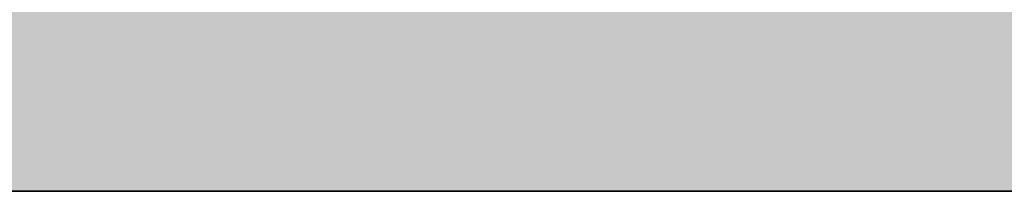
# Model space of a CAD drawing. Units: inches. Extents: x 2083 to 3317, y 1141 to 2115.
# Tile 138 of 256: x 3126.1318 to 3126.6699, y 1263.2614 to 1263.3548. Entities that reach past the tile are written whole.
import ezdxf

# ---------------------------------------------------------------- set-up
doc = ezdxf.new("R2010")
doc.units = ezdxf.units.IN
doc.layers.add('A-ANNO-DIMS', color=2, linetype='Continuous', lineweight=18)
doc.layers.add('A-WALL', color=7, linetype='Continuous', lineweight=35)
doc.layers.add('A-WALL-PATT', color=251, linetype='Continuous', lineweight=13, true_color=0x636466)
doc.styles.get("Standard").update_dxf_attribs({"font": 'arial.ttf'})
doc.dimstyles.new('ISO-25', dxfattribs={"dimtxt": 12, "dimasz": 12, "dimexe": 1.25, "dimexo": 0.625, "dimtad": 1, "dimlunit": 3, "dimtxsty": 'Standard', "dimcen": 2.5, "dimadec": 0, "dimazin": 0, "dimtfac": 1, "dimtmove": 0, "dimatfit": 3, "dimfxl": 1, "dimarcsym": 0})

# ---------------------------------------------------------------- blocks, each defined once
blk = doc.blocks.new('*D10')
at = {"layer": 'A-ANNO-DIMS', "color": 0, "lineweight": -2, "transparency": 16777216}
for p, q in [((2862.95978, 1262.63636), (2862.95978, 1201.38445)), ((3126.95978, 1262.63636), (3126.95978, 1201.38445)), ((2874.95978, 1202.63445), (3114.95978, 1202.63445))]:
    blk.add_line(p, q, dxfattribs=at)
at = {"layer": 'A-ANNO-DIMS', "color": 0, "transparency": 16777216}
for points in [[(2874.95978, 1204.63445), (2874.95978, 1200.63445), (2862.95978, 1202.63445)], [(3114.95978, 1204.63445), (3114.95978, 1200.63445), (3126.95978, 1202.63445)]]:
    blk.add_solid(points, dxfattribs=at)
at = {"layer": 'Defpoints', "color": 0, "transparency": 16777216}
for p in [(2862.95978, 1263.26136), (3126.95978, 1263.26136), (3126.95978, 1202.63445)]:
    blk.add_point(p, dxfattribs=at)
at = {"layer": 'A-ANNO-DIMS', "color": 0, "transparency": 16777216, "insert": (2994.95978, 1209.28401), "char_height": 12, "attachment_point": 5}
blk.add_mtext("22'", dxfattribs=at)
blk = doc.blocks.new('*D26')
at = {"layer": 'A-ANNO-DIMS', "color": 0, "lineweight": -2, "transparency": 16777216}
for p, q in [((3088.98584, 1274.91509), (3088.98584, 1270.95196)), ((3111.24004, 1274.91509), (3111.24004, 1270.95196)), ((3076.98584, 1272.20196), (2840.26245, 1272.20196)), ((3111.24004, 1272.20196), (3088.98584, 1272.20196)), ((3123.24004, 1272.20196), (3135.24004, 1272.20196))]:
    blk.add_line(p, q, dxfattribs=at)
at = {"layer": 'A-ANNO-DIMS', "color": 0, "transparency": 16777216}
for points in [[(3076.98584, 1274.20196), (3076.98584, 1270.20196), (3088.98584, 1272.20196)], [(3123.24004, 1274.20196), (3123.24004, 1270.20196), (3111.24004, 1272.20196)]]:
    blk.add_solid(points, dxfattribs=at)
at = {"layer": 'Defpoints', "color": 0, "transparency": 16777216}
for p in [(3088.98584, 1275.54009), (3111.24004, 1275.54009), (3088.98584, 1272.20196)]:
    blk.add_point(p, dxfattribs=at)
at = {"layer": 'A-ANNO-DIMS', "color": 0, "transparency": 16777216, "insert": (2952.62415, 1279.0316), "char_height": 12, "attachment_point": 5}
blk.add_mtext('NIGHTSTAND 1\'-10 1/2" TYP.', dxfattribs=at)
blk = doc.blocks.new('*D27')
at = {"layer": 'A-ANNO-DIMS', "color": 0, "lineweight": -2, "transparency": 16777216}
for p, q in [((3114.57817, 1309.79428), (3114.57817, 1321.79428)), ((3111.86504, 1297.79428), (3115.82817, 1297.79428)), ((3114.57817, 1297.79428), (3114.57817, 1275.54009)), ((3111.86504, 1275.54009), (3115.82817, 1275.54009)), ((3114.57817, 1263.54009), (3114.57817, 1140.98859))]:
    blk.add_line(p, q, dxfattribs=at)
at = {"layer": 'A-ANNO-DIMS', "color": 0, "transparency": 16777216}
for points in [[(3112.57817, 1309.79428), (3116.57817, 1309.79428), (3114.57817, 1297.79428)], [(3112.57817, 1263.54009), (3116.57817, 1263.54009), (3114.57817, 1275.54009)]]:
    blk.add_solid(points, dxfattribs=at)
at = {"layer": 'Defpoints', "color": 0, "transparency": 16777216}
for p in [(3111.24004, 1297.79428), (3111.24004, 1275.54009), (3114.57817, 1275.54009)]:
    blk.add_point(p, dxfattribs=at)
at = {"layer": 'A-ANNO-DIMS', "color": 0, "transparency": 16777216, "insert": (3107.74853, 1196.26434), "char_height": 12, "attachment_point": 5, "rotation": 90}
blk.add_mtext('1\'-10 1/2" TYP.', dxfattribs=at)

msp = doc.modelspace()

# ---------------------------------------------------------------- hatches: boundary and pattern name
at = {"layer": 'A-WALL-PATT'}
h = msp.add_hatch(color=256, dxfattribs=at)
h.dxf.hatch_style = 1
h.paths.add_polyline_path([(3126.95978, 2020.76136), (2748.95978, 2020.76136), (2604.95978, 2020.76136), (2226.95978, 2020.76136), (2226.95978, 1702.76136), (2466.95978, 1702.76136), (2466.95978, 1582.76136), (2418.95978, 1582.76136), (2418.95978, 1477.76136), (2226.95978, 1477.76136), (2226.95978, 1263.26136), (2544.95978, 1263.26136), (2544.95978, 1411.76136), (2604.95978, 1411.76136), (2685.95978, 1411.76136), (2685.95978, 1420.76136), (2604.95978, 1420.76136), (2604.95978, 1573.76136), (2604.95978, 1702.76136), (2604.95978, 2011.76136), (2748.95978, 2011.76136), (2748.95978, 1702.76136), (2862.95978, 1702.76136), (2862.95978, 1621.76136), (2871.95978, 1621.76136), (2871.95978, 1702.76136), (2883.95978, 1702.76136), (2883.95978, 1706.93946, -0.026459), (2883.95978, 1711.76136), (2757.95978, 1711.76136), (2757.95978, 1807.76136), (2787.95978, 1807.76136), (2787.95978, 1812.26136), (2757.95978, 1812.26136), (2757.95978, 2011.76136), (2877.95978, 2011.76136), (2877.95978, 1812.26136), (2847.95978, 1812.26136), (2847.95978, 1807.76136), (2889.83574, 1807.76136), (2889.83574, 1812.26136), (2882.45978, 1812.26136), (2882.45978, 2011.76136), (3117.95978, 2011.76136), (3117.95978, 1812.26136), (2937.83574, 1812.26136), (2937.83574, 1807.76136), (2995.70978, 1807.76136), (2995.70978, 1796.11767), (3000.20978, 1796.11767), (3000.20978, 1807.76136), (3117.95978, 1807.76136), (3117.95978, 1711.76136), (3000.20978, 1711.76136), (3000.20978, 1760.11767), (2998.5727, 1760.11767, -0.020711), (2995.70978, 1760.11767), (2995.70978, 1711.76136), (2931.95978, 1711.76136), (2931.95978, 1702.76136), (3126.95978, 1702.76136)])
h.paths.add_polyline_path([(2471.45978, 2011.76136), (2471.45978, 1810.01136), (2462.71694, 1810.01136), (2462.71694, 1805.51136), (2505.95978, 1805.51136), (2505.95978, 1810.01136), (2475.95978, 1810.01136), (2475.95978, 2011.76136), (2595.95978, 2011.76136), (2595.95978, 1810.01136), (2565.95978, 1810.01136), (2565.95978, 1805.51136), (2595.95978, 1805.51136), (2595.95978, 1711.76136), (2235.95978, 1711.76136), (2235.95978, 1805.51136), (2353.70978, 1805.51136), (2353.70978, 1796.05416), (2358.20978, 1796.05416), (2358.20978, 1805.51136), (2414.71694, 1805.51136), (2414.71694, 1810.01136), (2235.95978, 1810.01136), (2235.95978, 2011.76136)], flags=16)
h.paths.add_polyline_path([(2270.20473, 1994.61001), (2270.20473, 1970.61001), (2246.20473, 1970.61001), (2246.20473, 1994.61001)], flags=0)
edge = h.paths.add_edge_path(flags=0)
edge.add_ellipse((2332.02739, 1899.79818), major_axis=(-3.04299, 3.04299), ratio=0.1682525, start_angle=-161.33217, end_angle=-156.30711, ccw=False)
edge.add_ellipse((2333.08204, 1898.74353), major_axis=(-1.05465, 1.05465), ratio=0.4535321, start_angle=-123.37102, end_angle=-94.15911)
edge = h.paths.add_edge_path(flags=0)
edge.add_ellipse((2332.02739, 1968.87629), major_axis=(3.04299, 3.04299), ratio=0.1682525, start_angle=18.66783, end_angle=23.69289)
edge.add_spline(control_points=[(2332.9256, 1970.6911), (2332.22677, 1970.3361), (2330.89371, 1969.65891), (2328.41308, 1970.93214), (2327.20393, 1967.74871), (2324.7096, 1969.95559), (2322.53282, 1967.01235), (2320.01285, 1971.29581), (2317.68031, 1968.15784), (2316.04053, 1967.10205), (2315.4269, 1966.8096)], knot_values=[0, 0, 0, 0, 2.267059, 4.324559, 6.685584, 8.878641, 11.121502, 14.300359, 17.755284, 19.732645, 19.732645, 19.732645, 19.732645], degree=3, periodic=0)
edge.add_ellipse((2332.02739, 1968.87629), major_axis=(3.04299, 3.04299), ratio=0.1682525, start_angle=18.66783, end_angle=23.69289, ccw=False)
edge.add_ellipse((2333.08204, 1969.93094), major_axis=(1.05465, 1.05465), ratio=0.4535321, start_angle=56.62898, end_angle=85.84089, ccw=False)
edge = h.paths.add_edge_path(flags=0)
edge.add_spline(control_points=[(2296.42829, 1967.98791), (2293.6278, 1965.33631), (2287.70362, 1959.72709), (2299.74386, 1949.9957), (2294.53259, 1935.66853), (2290.57323, 1920.60351), (2293.39412, 1909.97369), (2296.18541, 1904.96654)], knot_values=[0.099185, 0.099185, 0.099185, 0.099185, 0.345301, 0.619822, 0.982653, 1.386093, 1.810555, 1.810555, 1.810555, 1.810555], degree=3, periodic=0)
edge.add_spline(control_points=[(2296.18541, 1904.96654), (2297.38358, 1902.6193), (2298.00097, 1901.94931), (2298.55297, 1901.46815)], knot_values=[0.006246, 0.006246, 0.006246, 0.006246, 0.055476, 0.055476, 0.055476, 0.055476], degree=3, periodic=0)
edge.add_spline(control_points=[(2298.55297, 1901.46815), (2297.25861, 1900.92322), (2295.22529, 1900.23213), (2293.06023, 1900.61421), (2292.10142, 1900.78841), (2292.08958, 1900.79057)], knot_values=[0.312835, 0.312835, 0.312835, 0.312835, 0.40178, 0.474987, 0.475903, 0.475903, 0.475903, 0.475903], degree=3, periodic=0)
edge.add_arc((2292.79365, 1904.66411), 3.93701, 215.4209, 259.69818, ccw=False)
edge.add_spline(control_points=[(2289.58531, 1902.3823), (2289.47665, 1902.53509), (2289.36848, 1902.68804), (2289.26086, 1902.84117)], knot_values=[0.102872, 0.102872, 0.102872, 0.102872, 0.116896, 0.116896, 0.116896, 0.116896], degree=3, periodic=0)
edge.add_spline(control_points=[(2289.26086, 1902.84117), (2288.6866, 1902.55019), (2287.64005, 1902.0199), (2285.88134, 1901.87395), (2283.85297, 1901.50435), (2281.71999, 1899.71054), (2278.46699, 1899.49294), (2276.15714, 1901.8832), (2272.25895, 1899.80407), (2267.77761, 1901.84318), (2262.24388, 1900.18403), (2257.41493, 1901.78206), (2254.31837, 1900.72612), (2253.17828, 1900.33734)], knot_values=[0, 0, 0, 0, 1.907977, 3.477176, 5.261074, 7.972851, 11.680248, 13.717921, 16.939592, 22.789562, 27.502503, 33.595215, 37.145618, 37.145618, 37.145618, 37.145618], degree=3, periodic=0)
edge.add_line((2253.17828, 1900.33734), (2250.24424, 1902.84117))
edge.add_line((2250.24424, 1902.84117), (2250.24424, 1965.8333))
edge.add_line((2250.24424, 1965.8333), (2253.17828, 1968.33712))
edge.add_spline(control_points=[(2253.17828, 1968.33712), (2254.31837, 1967.94835), (2257.41493, 1966.89241), (2262.24388, 1968.49043), (2267.77761, 1966.83128), (2271.52673, 1968.53722), (2273.87591, 1967.82829), (2274.2067, 1967.72764)], knot_values=[0, 0, 0, 0, 0.09018, 0.244935, 0.364644, 0.513233, 0.537855, 0.537855, 0.537855, 0.537855], degree=3, periodic=0)
edge.add_arc((2274.35289, 1963.79335), 3.93701, 72.05113, 92.12795, ccw=False)
edge.add_arc((2281.29693, 1985.23), 18.5963, 252.051134, 288.565722)
edge.add_arc((2292.31672, 1956.02888), 12.64608, 71.026788, 113.778218, ccw=False)
edge = h.paths.add_edge_path(flags=0)
edge.add_spline(control_points=[(2274.89941, 1951.85619), (2275.06616, 1951.61659), (2275.23269, 1951.37659), (2275.39799, 1951.13585)], knot_values=[1.409916, 1.409916, 1.409916, 1.409916, 1.43159, 1.43159, 1.43159, 1.43159], degree=3, periodic=0)
edge.add_spline(control_points=[(2275.39799, 1951.13585), (2275.79211, 1950.56189), (2276.17923, 1949.98377), (2276.54555, 1949.3971)], knot_values=[1.358238, 1.358238, 1.358238, 1.358238, 1.409916, 1.409916, 1.409916, 1.409916], degree=3, periodic=0)
edge.add_line((2276.54555, 1949.3971), (2277.43729, 1947.86218))
edge.add_spline(control_points=[(2277.43729, 1947.86218), (2276.30383, 1945.67311), (2274.6397, 1942.42688), (2274.63161, 1938.0939), (2272.79912, 1930.85155), (2274.35643, 1943.89705), (2275.94768, 1947.92336), (2276.54555, 1949.3971)], knot_values=[0.005632, 0.005632, 0.005632, 0.005632, 0.186014, 0.266002, 0.357087, 0.59639, 0.739732, 0.739732, 0.739732, 0.739732], degree=3, periodic=0)
edge.add_spline(control_points=[(2276.54555, 1949.3971), (2276.17923, 1949.98377), (2275.79211, 1950.56189), (2275.39799, 1951.13585)], knot_values=[1.358238, 1.358238, 1.358238, 1.358238, 1.409916, 1.409916, 1.409916, 1.409916], degree=3, periodic=0)
edge.add_spline(control_points=[(2275.39799, 1951.13585), (2274.9425, 1950.08045), (2274.20776, 1948.02527), (2273.9346, 1944.85148), (2272.46853, 1937.62749), (2273.46622, 1945.69647), (2274.70062, 1951.05947), (2274.89941, 1951.85619)], knot_values=[0.104364, 0.104364, 0.104364, 0.104364, 0.189636, 0.269624, 0.36071, 0.600013, 0.644622, 0.644622, 0.644622, 0.644622], degree=3, periodic=0)
h.paths.add_polyline_path([(2269.16751, 1963.12757, -0.357527), (2268.17063, 1960.97637, -0.092561), (2268.17063, 1939.43632, -0.357527), (2269.16751, 1937.28512, -0.357527), (2267.01631, 1938.282, -0.164785), (2254.68558, 1938.282, -0.357527), (2252.53438, 1937.28512, -0.357527), (2253.53126, 1939.43632, -0.092561), (2253.53126, 1960.97637, -0.357527), (2252.53438, 1963.12757, -0.357527), (2254.68558, 1962.13069, -0.164785), (2267.01631, 1962.13069, -0.357527)], flags=0)
h.paths.add_polyline_path([(2248.87407, 1967.8018), (2248.87407, 1957.02771), (2249.45778, 1957.02771), (2249.45778, 1911.64676), (2248.87407, 1911.64676), (2248.87407, 1900.87267), (2246.51186, 1900.87267, 0.197327), (2244.14966, 1902.45687), (2244.14966, 1966.21759, 0.197327), (2246.51186, 1967.8018)], flags=0)
h.paths.add_polyline_path([(2269.16751, 1931.38934, -0.357527), (2268.17063, 1929.23814, -0.092561), (2268.17063, 1907.6981, -0.357527), (2269.16751, 1905.54689, -0.357527), (2267.01631, 1906.54377, -0.164785), (2254.68558, 1906.54377, -0.357527), (2252.53438, 1905.54689, -0.357527), (2253.53126, 1907.6981, -0.092561), (2253.53126, 1929.23814, -0.357527), (2252.53438, 1931.38934, -0.357527), (2254.68558, 1930.39246, -0.164785), (2267.01631, 1930.39246, -0.357527)], flags=0)
edge = h.paths.add_edge_path(flags=0)
edge.add_spline(control_points=[(2276.19686, 1906.7237), (2276.16814, 1909.02893), (2276.11405, 1913.37185), (2270.59842, 1924.92498), (2273.90517, 1919.01278), (2275.92171, 1916.26206), (2275.47457, 1912.40215), (2277.25787, 1910.38062), (2276.69604, 1908.22504), (2276.64622, 1906.81302), (2276.61782, 1906.00841)], knot_values=[0, 0, 0, 0, 8.61026, 16.221274, 18.843057, 23.804898, 27.440828, 29.356102, 31.203478, 33.650687, 33.650687, 33.650687, 33.650687], degree=3, periodic=0)
edge.add_spline(control_points=[(2276.61782, 1906.00841), (2276.62331, 1905.62414), (2276.49774, 1904.62866), (2275.44178, 1903.85473), (2274.93731, 1903.08045), (2274.85908, 1902.84117)], knot_values=[0.156488, 0.156488, 0.156488, 0.156488, 0.184398, 0.231376, 0.250598, 0.250598, 0.250598, 0.250598], degree=3, periodic=0)
edge.add_line((2274.85908, 1902.84117), (2276.50598, 1902.84117))
edge.add_spline(control_points=[(2276.50598, 1902.84117), (2276.78831, 1903.08494), (2277.66507, 1904.1252), (2278.24954, 1904.34074), (2277.65387, 1908.52739), (2278.15567, 1906.22781), (2278.10046, 1905.28595), (2278.84667, 1904.06901), (2277.85679, 1903.41495), (2277.87419, 1902.99105), (2277.90356, 1902.84117)], knot_values=[0.059574, 0.059574, 0.059574, 0.059574, 0.080753, 0.103741, 0.16972, 0.176036, 0.207137, 0.240474, 0.262341, 0.27366, 0.27366, 0.27366, 0.27366], degree=3, periodic=0)
edge.add_line((2277.90356, 1902.84117), (2280.02983, 1902.84117))
edge.add_spline(control_points=[(2280.02983, 1902.84117), (2279.88822, 1903.0884), (2279.49926, 1903.98155), (2280.15228, 1905.93935), (2278.10362, 1909.65776), (2279.76239, 1907.18529), (2280.3279, 1904.87486), (2280.48511, 1903.48959), (2281.46327, 1903.24943), (2281.75834, 1902.9365), (2281.83404, 1902.84117)], knot_values=[0.013856, 0.013856, 0.013856, 0.013856, 0.034874, 0.088867, 0.107879, 0.126738, 0.158714, 0.193757, 0.217487, 0.226722, 0.226722, 0.226722, 0.226722], degree=3, periodic=0)
edge.add_spline(control_points=[(2281.83404, 1902.84117), (2281.78753, 1902.8267), (2281.64702, 1902.78299), (2281.39553, 1902.85949), (2281.08808, 1902.98524), (2280.72068, 1903.0609), (2280.33345, 1903.02573), (2280.12477, 1902.89888), (2280.02983, 1902.84117)], knot_values=[0, 0, 0, 0, 0.14413, 0.435517, 0.749276, 1.153046, 1.548371, 1.878348, 1.878348, 1.878348, 1.878348], degree=3, periodic=0)
edge.add_line((2280.02983, 1902.84117), (2277.90356, 1902.84117))
edge.add_spline(control_points=[(2277.90356, 1902.84117), (2277.89286, 1902.79586), (2277.8654, 1902.67964), (2277.60748, 1902.68748), (2277.27405, 1902.8007), (2276.83792, 1902.61977), (2276.58381, 1902.78926), (2276.50598, 1902.84117)], knot_values=[0, 0, 0, 0, 0.127189, 0.326199, 0.628009, 1.24357, 1.515331, 1.515331, 1.515331, 1.515331], degree=3, periodic=0)
edge.add_line((2276.50598, 1902.84117), (2274.85908, 1902.84117))
edge.add_spline(control_points=[(2274.85908, 1902.84117), (2274.81444, 1902.89859), (2274.72513, 1903.01345), (2274.49348, 1903.11897), (2274.24429, 1902.96054), (2273.93712, 1903.18494), (2273.61404, 1902.98314), (2273.40832, 1902.88304), (2273.32225, 1902.84117)], knot_values=[0, 0, 0, 0, 0.21843, 0.436957, 0.687977, 0.990379, 1.398396, 1.69185, 1.69185, 1.69185, 1.69185], degree=3, periodic=0)
edge.add_spline(control_points=[(2273.32225, 1902.84117), (2273.61674, 1903.44569), (2274.274, 1904.53825), (2276.02724, 1904.5737), (2276.20696, 1906.58364), (2276.19686, 1906.7237)], knot_values=[0.012227, 0.012227, 0.012227, 0.012227, 0.059472, 0.106218, 0.134458, 0.134458, 0.134458, 0.134458], degree=3, periodic=0)
h.paths.add_polyline_path([(2270.77605, 1897.78983), (2270.77605, 1873.78983), (2246.77605, 1873.78983), (2246.77605, 1897.78983)], flags=0)
h.paths.add_polyline_path([(2353.70978, 1760.00506), (2353.70978, 1760.05416), (2358.20978, 1760.05416, -0.033729)], flags=0)
h.paths.add_polyline_path([(2321.81912, 1737.52919), (2341.99533, 1737.52919, -0.414214), (2343.20327, 1736.32124), (2343.20327, 1721.0206, -0.414214), (2341.99533, 1719.81265), (2321.81912, 1719.81265, -0.414214), (2320.61117, 1721.0206), (2320.61117, 1736.32124, -0.414214)], flags=0)
h.paths.add_polyline_path([(2324.23501, 1736.32124), (2339.57944, 1736.32124, -0.414214), (2341.99533, 1733.90535), (2341.99533, 1725.44973, -0.414214), (2339.57944, 1723.03384), (2333.68059, 1723.03384), (2333.84532, 1722.04547, -0.870646), (2335.4254, 1721.82589, -0.767327), (2333.92269, 1721.42324), (2331.29102, 1721.42324, -0.767327), (2329.78832, 1721.82589, -0.870646), (2331.3684, 1722.04547), (2331.53313, 1723.03384), (2324.23501, 1723.03384, -0.414214), (2321.81912, 1725.44973), (2321.81912, 1733.90535, -0.414214)], flags=0)
h.paths.add_polyline_path([(2570.48379, 1928.61544), (2589.68379, 1928.61544), (2590.16883, 1928.61544), (2590.16883, 1904.9934), (2570.48379, 1904.9934)], flags=0)
h.paths.add_polyline_path([(2574.44732, 1927.26382, -1), (2572.82884, 1927.26382, -1)], flags=0)
h.paths.add_polyline_path([(2573.08987, 1926.94088), (2573.92503, 1927.77604), (2574.14774, 1927.55333), (2573.31258, 1926.71817)], flags=0)
h.paths.add_polyline_path([(2578.77906, 1919.72962, -1), (2571.59166, 1919.72962, -1)], flags=0)
h.paths.add_polyline_path([(2578.38536, 1919.72962, -1), (2571.98536, 1919.72962, -1)], flags=0)
h.paths.add_polyline_path([(2331.59576, 1729.47622, -1), (2333.61795, 1729.47622, -1)], flags=0)
h.paths.add_polyline_path([(2578.03423, 1927.26382, -1), (2576.41574, 1927.26382, -1)], flags=0)
h.paths.add_polyline_path([(2576.68885, 1927.53109), (2576.91156, 1927.7538), (2577.74673, 1926.91863), (2577.52402, 1926.69592)], flags=0)
h.paths.add_polyline_path([(2578.13906, 1909.85954, -1), (2572.23166, 1909.85954, -1)], flags=0)
h.paths.add_polyline_path([(2577.74536, 1909.85954, -1), (2572.62536, 1909.85954, -1)], flags=0)
h.paths.add_polyline_path([(2583.79772, 1927.26382, -1), (2582.17923, 1927.26382, -1)], flags=0)
h.paths.add_polyline_path([(2582.71865, 1927.7538), (2583.55381, 1926.91863), (2583.3311, 1926.69592), (2582.49594, 1927.53109)], flags=0)
h.paths.add_polyline_path([(2582.49594, 1927.53109), (2582.71865, 1927.7538), (2583.55381, 1926.91863), (2583.3311, 1926.69592)], flags=0)
h.paths.add_polyline_path([(2587.73906, 1920.52962, -1), (2581.83166, 1920.52962, -1)], flags=0)
h.paths.add_polyline_path([(2587.34536, 1920.52962, -1), (2582.22536, 1920.52962, -1)], flags=0)
h.paths.add_polyline_path([(2587.38462, 1927.26382, -1), (2585.76613, 1927.26382, -1)], flags=0)
h.paths.add_polyline_path([(2586.08199, 1926.98025), (2586.91716, 1927.81541), (2587.13987, 1927.5927), (2586.3047, 1926.75754)], flags=0)
h.paths.add_polyline_path([(2588.37906, 1910.65954, -1), (2581.19166, 1910.65954, -1)], flags=0)
h.paths.add_polyline_path([(2587.98536, 1910.65954, -1), (2581.58536, 1910.65954, -1)], flags=0)
h.paths.add_polyline_path([(2417.16773, 1729.4779), (2437.34394, 1729.4779, -0.414214), (2438.55188, 1728.26995), (2438.55188, 1712.96931, -0.414214), (2437.34394, 1711.76136), (2417.16773, 1711.76136, -0.414214), (2415.95978, 1712.96931), (2415.95978, 1728.26995, -0.414214)], flags=0)
h.paths.add_polyline_path([(2419.58362, 1728.26995), (2434.92805, 1728.26995, -0.414214), (2437.34394, 1725.85406), (2437.34394, 1717.39844, -0.414214), (2434.92805, 1714.98255), (2429.0292, 1714.98255), (2429.19393, 1713.99418, -0.870646), (2430.77401, 1713.7746, -0.767327), (2429.2713, 1713.37195), (2426.63963, 1713.37195, -0.767327), (2425.13693, 1713.7746, -0.870646), (2426.71701, 1713.99418), (2426.88174, 1714.98255), (2419.58362, 1714.98255, -0.414214), (2417.16773, 1717.39844), (2417.16773, 1725.85406, -0.414214)], flags=0)
h.paths.add_polyline_path([(2419.58362, 1728.26995), (2434.92805, 1728.26995, -0.414214), (2437.34394, 1725.85406), (2437.34394, 1717.39844, -0.414214), (2434.92805, 1714.98255), (2429.0292, 1714.98255), (2428.35812, 1719.00903), (2427.55282, 1719.00903), (2426.88174, 1714.98255), (2419.58362, 1714.98255, -0.414214), (2417.16773, 1717.39844), (2417.16773, 1725.85406, -0.414214)], flags=0)
h.paths.add_polyline_path([(2426.94437, 1721.42492, -1), (2428.96656, 1721.42492, -1)], flags=0)
h.paths.add_polyline_path([(2475.95978, 1702.76136), (2595.95978, 1702.76136), (2595.95978, 1582.76136), (2475.95978, 1582.76136)], flags=16)
h.paths.add_polyline_path([(2427.95978, 1573.76136), (2595.95978, 1573.76136), (2595.95978, 1468.76136), (2595.95978, 1420.76136), (2384.45978, 1420.76136), (2384.45978, 1468.76136), (2427.95978, 1468.76136)], flags=16)
h.paths.add_polyline_path([(2379.95978, 1468.76136), (2379.95978, 1420.76136), (2235.95978, 1420.76136), (2235.95978, 1468.76136)], flags=16)
h.paths.add_polyline_path([(2317.816, 1466.69577), (2337.9922, 1466.69577, -0.414214), (2339.20015, 1465.48782), (2339.20015, 1450.18718, -0.414214), (2337.9922, 1448.97923), (2317.816, 1448.97923, -0.414214), (2316.60805, 1450.18718), (2316.60805, 1465.48782, -0.414214)], flags=0)
h.paths.add_polyline_path([(2320.23189, 1465.48782), (2335.57631, 1465.48782, -0.414214), (2337.9922, 1463.07193), (2337.9922, 1454.61631, -0.414214), (2335.57631, 1452.20042), (2329.67747, 1452.20042), (2329.84219, 1451.21205, -0.870646), (2331.42228, 1450.99247, -0.767327), (2329.91957, 1450.58983), (2327.2879, 1450.58983, -0.767327), (2325.7852, 1450.99247, -0.870646), (2327.36528, 1451.21205), (2327.53001, 1452.20042), (2320.23189, 1452.20042, -0.414214), (2317.816, 1454.61631), (2317.816, 1463.07193, -0.414214)], flags=0)
h.paths.add_polyline_path([(2320.23189, 1465.48782), (2335.57631, 1465.48782, -0.414214), (2337.9922, 1463.07193), (2337.9922, 1454.61631, -0.414214), (2335.57631, 1452.20042), (2329.67747, 1452.20042), (2329.00638, 1456.22691), (2328.20109, 1456.22691), (2327.53001, 1452.20042), (2320.23189, 1452.20042, -0.414214), (2317.816, 1454.61631), (2317.816, 1463.07193, -0.414214)], flags=0)
h.paths.add_polyline_path([(2327.59264, 1458.6428, -1), (2329.61483, 1458.6428, -1)], flags=0)
h.paths.add_polyline_path([(2244.41174, 1433.34045), (2241.92094, 1433.34045, -0.414214), (2240.01786, 1435.24354), (2240.01786, 1440.95281, -0.414211), (2241.92093, 1442.8559), (2244.41174, 1442.8559, -1.976472)], flags=0)
h.paths.add_polyline_path([(2245.35689, 1434.39754, -0.414214), (2245.35689, 1441.79881, -2.144098)], flags=0)
h.paths.add_polyline_path([(2535.95978, 1416.26136), (2535.95978, 1272.26136), (2235.95978, 1272.26136), (2235.95978, 1416.26136)], flags=16)
h.paths.add_polyline_path([(2260.11956, 1384.29284), (2260.11956, 1362.03865), (2237.86537, 1362.03865), (2237.86537, 1384.29284)], flags=0)
edge = h.paths.add_edge_path(flags=0)
edge.add_line((2318.25185, 1362.0933), (2318.1458, 1362.00097))
edge.add_ellipse((2317.44512, 1360.43104), major_axis=(2.82164, 2.82164), ratio=0.1682525, start_angle=18.66783, end_angle=20.94813, ccw=False)
edge.add_ellipse((2318.42305, 1361.40897), major_axis=(0.97793, 0.97793), ratio=0.4535321, start_angle=56.62898, end_angle=70.2262, ccw=False)
edge = h.paths.add_edge_path(flags=0)
edge.add_line((2319.10737, 1295.57108), (2319.01504, 1295.67713))
edge.add_ellipse((2317.44512, 1296.37781), major_axis=(-2.82164, 2.82164), ratio=0.1682525, start_angle=-161.33217, end_angle=-159.05187, ccw=False)
edge.add_ellipse((2318.42305, 1295.39988), major_axis=(-0.97793, 0.97793), ratio=0.4535321, start_angle=-123.37102, end_angle=-109.7738)
edge = h.paths.add_edge_path(flags=0)
edge.add_spline(control_points=[(2284.21035, 1301.17022), (2284.58069, 1300.44472), (2284.89119, 1299.89202), (2285.15955, 1299.46102)], knot_values=[0.039066, 0.039066, 0.039066, 0.039066, 0.055476, 0.055476, 0.055476, 0.055476], degree=3, periodic=0)
edge.add_line((2285.15955, 1299.46102), (2284.21035, 1301.17022))
edge = h.paths.add_edge_path(flags=0)
edge.add_line((2280.41246, 1297.29801), (2283.36999, 1297.03612))
edge.add_line((2283.36999, 1297.03612), (2286.40569, 1297.92631))
edge.add_spline(control_points=[(2286.40569, 1297.92631), (2285.30549, 1297.46312), (2284.34478, 1297.12915), (2283.36999, 1297.03612)], knot_values=[0.394369, 0.394369, 0.394369, 0.394369, 0.475903, 0.475903, 0.475903, 0.475903], degree=3, periodic=0)
edge.add_spline(control_points=[(2283.36999, 1297.03612), (2283.28139, 1297.02767), (2282.31629, 1296.95734), (2281.3125, 1297.13448), (2280.42344, 1297.29602), (2280.41246, 1297.29801)], knot_values=[0.312835, 0.312835, 0.312835, 0.312835, 0.320246, 0.393453, 0.394369, 0.394369, 0.394369, 0.394369], degree=3, periodic=0)
edge = h.paths.add_edge_path(flags=0)
edge.add_line((2284.43556, 1359.60729), (2280.44629, 1355.32805))
edge.add_line((2280.44629, 1355.32805), (2279.57999, 1351.01775))
edge.add_line((2279.57999, 1351.01775), (2282.41297, 1346.58043))
edge.add_spline(control_points=[(2282.41297, 1346.58043), (2283.15333, 1345.58924), (2284.2529, 1344.0289), (2284.80104, 1342.38717), (2284.93516, 1341.80554)], knot_values=[1.240098, 1.240098, 1.240098, 1.240098, 1.332892, 1.382712, 1.382712, 1.382712, 1.382712], degree=3, periodic=0)
edge.add_spline(control_points=[(2284.93516, 1341.80554), (2285.31911, 1340.1406), (2285.23303, 1338.4092), (2284.90994, 1336.65412)], knot_values=[1.097484, 1.097484, 1.097484, 1.097484, 1.240098, 1.240098, 1.240098, 1.240098], degree=3, periodic=0)
edge.add_spline(control_points=[(2284.90994, 1336.65412), (2284.58685, 1334.89904), (2284.02675, 1333.12027), (2283.46264, 1331.36058)], knot_values=[0.95487, 0.95487, 0.95487, 0.95487, 1.097484, 1.097484, 1.097484, 1.097484], degree=3, periodic=0)
edge.add_line((2283.46264, 1331.36058), (2281.89038, 1326.15336))
edge.add_line((2281.89038, 1326.15336), (2280.75626, 1321.05609))
edge.add_line((2280.75626, 1321.05609), (2280.2992, 1316.00198))
edge.add_line((2280.2992, 1316.00198), (2280.71593, 1310.95007))
edge.add_line((2280.71593, 1310.95007), (2282.02809, 1305.97214))
edge.add_line((2282.02809, 1305.97214), (2284.21035, 1301.17022))
edge.add_spline(control_points=[(2284.21035, 1301.17022), (2283.34073, 1302.73019), (2282.6119, 1304.33649), (2282.02809, 1305.97214)], knot_values=[0.099185, 0.099185, 0.099185, 0.099185, 0.241799, 0.241799, 0.241799, 0.241799], degree=3, periodic=0)
edge.add_spline(control_points=[(2282.02809, 1305.97214), (2281.44428, 1307.60778), (2281.00549, 1309.27276), (2280.71593, 1310.95007)], knot_values=[0.241799, 0.241799, 0.241799, 0.241799, 0.384413, 0.384413, 0.384413, 0.384413], degree=3, periodic=0)
edge.add_spline(control_points=[(2280.71593, 1310.95007), (2280.43324, 1312.58761), (2280.28939, 1314.27696), (2280.29889, 1315.96203), (2280.2992, 1316.00198)], knot_values=[0.384413, 0.384413, 0.384413, 0.384413, 0.523647, 0.527028, 0.527028, 0.527028, 0.527028], degree=3, periodic=0)
edge.add_spline(control_points=[(2280.2992, 1316.00198), (2280.31233, 1317.68696), (2280.47787, 1319.36793), (2280.75626, 1321.05609)], knot_values=[0.527028, 0.527028, 0.527028, 0.527028, 0.669642, 0.669642, 0.669642, 0.669642], degree=3, periodic=0)
edge.add_spline(control_points=[(2280.75626, 1321.05609), (2281.03465, 1322.74425), (2281.42588, 1324.43961), (2281.89038, 1326.15336)], knot_values=[0.669642, 0.669642, 0.669642, 0.669642, 0.812256, 0.812256, 0.812256, 0.812256], degree=3, periodic=0)
edge.add_spline(control_points=[(2281.89038, 1326.15336), (2282.26438, 1327.53325), (2282.78787, 1329.26181), (2283.35275, 1331.01778), (2283.46264, 1331.36058)], knot_values=[0.812256, 0.812256, 0.812256, 0.812256, 0.927087, 0.95487, 0.95487, 0.95487, 0.95487], degree=3, periodic=0)
edge.add_line((2283.46264, 1331.36058), (2284.90994, 1336.65412))
edge.add_line((2284.90994, 1336.65412), (2284.93516, 1341.80554))
edge.add_line((2284.93516, 1341.80554), (2282.41297, 1346.58043))
edge.add_spline(control_points=[(2282.41297, 1346.58043), (2281.27513, 1348.10379), (2280.07845, 1349.57032), (2279.57999, 1351.01775)], knot_values=[1.382712, 1.382712, 1.382712, 1.382712, 1.525326, 1.525326, 1.525326, 1.525326], degree=3, periodic=0)
edge.add_spline(control_points=[(2279.57999, 1351.01775), (2279.44328, 1351.41472), (2279.13631, 1352.85692), (2279.73519, 1354.29039), (2280.44629, 1355.32805)], knot_values=[1.525326, 1.525326, 1.525326, 1.525326, 1.564439, 1.667941, 1.667941, 1.667941, 1.667941], degree=3, periodic=0)
edge.add_spline(control_points=[(2280.44629, 1355.32805), (2281.42611, 1356.75784), (2282.93084, 1358.18256), (2284.43556, 1359.60729)], knot_values=[1.667941, 1.667941, 1.667941, 1.667941, 1.810555, 1.810555, 1.810555, 1.810555], degree=3, periodic=0)
edge.add_arc((2280.62307, 1348.51818), 11.72618, 71.026788, 113.778218)
edge.add_arc((2270.40489, 1375.59516), 17.24357, 252.051134, 288.565722, ccw=False)
edge.add_arc((2263.96597, 1355.71785), 3.65062, 72.05113, 92.12795)
edge.add_arc((2263.96597, 1355.71785), 3.65062, 92.12795, 177.98513)
edge.add_spline(control_points=[(2260.3176, 1355.8462), (2260.26042, 1354.22067), (2260.55128, 1350.18655), (2262.99934, 1346.76625), (2264.47274, 1344.64902)], knot_values=[1.43159, 1.43159, 1.43159, 1.43159, 1.564144, 1.770695, 1.770695, 1.770695, 1.770695], degree=3, periodic=0)
edge.add_line((2264.47274, 1344.64902), (2264.93559, 1343.98253))
edge.add_spline(control_points=[(2263.80104, 1340.24811), (2263.84324, 1340.51409), (2264.06724, 1341.75647), (2264.51269, 1343.00245), (2264.93505, 1343.98108)], knot_values=[0.53657, 0.53657, 0.53657, 0.53657, 0.559349, 0.644622, 0.644622, 0.644622, 0.644622], degree=3, periodic=0)
edge.add_spline(control_points=[(2264.93505, 1343.98108), (2265.11777, 1343.71497), (2265.29888, 1343.44791), (2265.47676, 1343.17936)], knot_values=[1.384077, 1.384077, 1.384077, 1.384077, 1.409916, 1.409916, 1.409916, 1.409916], degree=3, periodic=0)
edge.add_spline(control_points=[(2265.47676, 1343.17936), (2265.65464, 1342.91082), (2265.8293, 1342.64081), (2265.99913, 1342.36881)], knot_values=[1.358238, 1.358238, 1.358238, 1.358238, 1.384077, 1.384077, 1.384077, 1.384077], degree=3, periodic=0)
edge.add_line((2265.99913, 1342.36881), (2266.82601, 1340.94555))
edge.add_spline(control_points=[(2266.82601, 1340.94555), (2268.8944, 1337.08969), (2271.39817, 1325.843), (2270.51616, 1310.56856), (2275.91938, 1301.86061), (2277.78951, 1299.19945)], knot_values=[0.116896, 0.116896, 0.116896, 0.116896, 0.472987, 1.050969, 1.313793, 1.313793, 1.313793, 1.313793], degree=3, periodic=0)
edge.add_spline(control_points=[(2277.78951, 1299.19945), (2277.83941, 1299.12845), (2277.88943, 1299.0575), (2277.93957, 1298.98658)], knot_values=[0.109884, 0.109884, 0.109884, 0.109884, 0.116896, 0.116896, 0.116896, 0.116896], degree=3, periodic=0)
edge.add_line((2277.93957, 1298.98658), (2277.78885, 1299.19911))
edge.add_spline(control_points=[(2277.78885, 1299.19911), (2277.25658, 1298.92941), (2276.28635, 1298.4379), (2275.03935, 1298.33442), (2274.38333, 1298.2389), (2274.21525, 1298.20934)], knot_values=[33.12187, 33.12187, 33.12187, 33.12187, 35.029056, 36.598255, 37.144827, 37.144827, 37.144827, 37.144827], degree=3, periodic=0)
edge.add_line((2274.21525, 1298.20934), (2273.07315, 1297.89296))
edge.add_spline(control_points=[(2273.07315, 1297.89296), (2272.32294, 1297.57978), (2271.03915, 1296.51051), (2269.24839, 1296.22606), (2268.4231, 1296.37465)], knot_values=[26.532584, 26.532584, 26.532584, 26.532584, 29.198919, 31.839101, 31.839101, 31.839101, 31.839101], degree=3, periodic=0)
edge.add_line((2268.4231, 1296.37465), (2263.8785, 1297.45753))
edge.add_spline(control_points=[(2263.8785, 1297.45753), (2263.55608, 1297.35943), (2261.86031, 1296.83869), (2260.23878, 1297.28241), (2258.93345, 1297.51646)], knot_values=[15.919551, 15.919551, 15.919551, 15.919551, 16.939592, 21.226067, 21.226067, 21.226067, 21.226067], degree=3, periodic=0)
edge.add_line((2258.93345, 1297.51646), (2254.05523, 1297.32901))
edge.add_spline(control_points=[(2254.05523, 1297.32901), (2253.75553, 1297.29582), (2252.11368, 1297.16517), (2250.46187, 1297.54422), (2249.12969, 1297.66788)], knot_values=[5.306517, 5.306517, 5.306517, 5.306517, 6.276435, 10.613034, 10.613034, 10.613034, 10.613034], degree=3, periodic=0)
edge.add_line((2249.12969, 1297.66788), (2244.33165, 1296.87776))
edge.add_line((2244.33165, 1296.87776), (2241.61103, 1299.19945))
edge.add_line((2241.61103, 1299.19945), (2241.61103, 1357.6094))
edge.add_line((2241.61103, 1357.6094), (2244.33165, 1359.9311))
edge.add_line((2244.33165, 1359.9311), (2252.72882, 1359.54269))
edge.add_spline(control_points=[(2252.72882, 1359.54269), (2252.87094, 1359.54644), (2253.30574, 1359.54817), (2253.73984, 1359.51427), (2254.03174, 1359.48243)], knot_values=[0.233291, 0.233291, 0.233291, 0.233291, 0.244935, 0.268927, 0.268927, 0.268927, 0.268927], degree=3, periodic=0)
edge.add_line((2254.03174, 1359.48243), (2259.58719, 1359.41639))
edge.add_spline(control_points=[(2259.58719, 1359.41639), (2260.67707, 1359.6285), (2262.0732, 1359.897), (2263.52369, 1359.45928), (2263.83042, 1359.36595)], knot_values=[0.422516, 0.422516, 0.422516, 0.422516, 0.513233, 0.537855, 0.537855, 0.537855, 0.537855], degree=3, periodic=0)
edge.add_arc((2263.96597, 1355.71785), 3.65062, 72.05113, 92.12795, ccw=False)
edge.add_arc((2270.40489, 1375.59516), 17.24357, 252.051134, 288.565722)
edge.add_arc((2280.62307, 1348.51818), 11.72618, 71.026788, 113.778218, ccw=False)
h.paths.add_polyline_path([(2240.34053, 1359.43471), (2240.34053, 1349.44435), (2240.88178, 1349.44435), (2240.88178, 1307.3645), (2240.34053, 1307.3645), (2240.34053, 1297.37414), (2238.15016, 1297.37414, 0.197327), (2235.95978, 1298.84311), (2235.95978, 1357.96575, 0.197327), (2238.15016, 1359.43471)], flags=0)
h.paths.add_polyline_path([(2259.15779, 1355.1005, -0.357527), (2258.23342, 1353.10578, -0.092561), (2258.23342, 1333.1326, -0.357527), (2259.15779, 1331.13788, -0.357527), (2257.16307, 1332.06225, -0.164785), (2245.7293, 1332.06225, -0.357527), (2243.73458, 1331.13788, -0.357527), (2244.65895, 1333.1326, -0.092561), (2244.65895, 1353.10578, -0.357527), (2243.73458, 1355.1005, -0.357527), (2245.7293, 1354.17613, -0.164785), (2257.16307, 1354.17613, -0.357527)], flags=0)
edge = h.paths.add_edge_path(flags=0)
edge.add_line((2265.99913, 1342.36881), (2266.82601, 1340.94555))
edge.add_line((2266.82601, 1340.94555), (2265.30756, 1337.81407))
edge.add_line((2265.30756, 1337.81407), (2264.35823, 1334.65294))
edge.add_line((2264.35823, 1334.65294), (2264.26201, 1333.7997))
edge.add_spline(control_points=[(2264.26201, 1333.7997), (2264.20836, 1333.18705), (2264.16206, 1332.36553), (2264.00714, 1331.41393), (2263.96905, 1331.20183)], knot_values=[0.464444, 0.464444, 0.464444, 0.464444, 0.516691, 0.531608, 0.531608, 0.531608, 0.531608], degree=3, periodic=0)
edge.add_spline(control_points=[(2263.96905, 1331.20183), (2263.77453, 1330.11887), (2263.42437, 1328.79084), (2263.25742, 1328.53065), (2263.23403, 1328.51461)], knot_values=[0.372682, 0.372682, 0.372682, 0.372682, 0.44885, 0.464444, 0.464444, 0.464444, 0.464444], degree=3, periodic=0)
edge.add_spline(control_points=[(2263.23403, 1328.51461), (2263.09638, 1328.42023), (2263.13117, 1329.30148), (2263.27495, 1330.61575)], knot_values=[0.280919, 0.280919, 0.280919, 0.280919, 0.372682, 0.372682, 0.372682, 0.372682], degree=3, periodic=0)
edge.add_spline(control_points=[(2263.27495, 1330.61575), (2263.41874, 1331.93002), (2263.67152, 1333.67732), (2263.96985, 1335.31503)], knot_values=[0.189157, 0.189157, 0.189157, 0.189157, 0.280919, 0.280919, 0.280919, 0.280919], degree=3, periodic=0)
edge.add_spline(control_points=[(2263.96985, 1335.31503), (2264.1005, 1336.03219), (2264.41878, 1337.62191), (2264.75485, 1338.86443), (2264.94742, 1339.49112)], knot_values=[0.097394, 0.097394, 0.097394, 0.097394, 0.137578, 0.189157, 0.189157, 0.189157, 0.189157], degree=3, periodic=0)
edge.add_spline(control_points=[(2264.94742, 1339.49112), (2265.29002, 1340.60605), (2265.64424, 1341.494), (2265.99913, 1342.36881)], knot_values=[0.005632, 0.005632, 0.005632, 0.005632, 0.097394, 0.097394, 0.097394, 0.097394], degree=3, periodic=0)
h.paths.add_polyline_path([(2259.15779, 1325.67097, -0.357527), (2258.23342, 1323.67625, -0.092561), (2258.23342, 1303.70307, -0.357527), (2259.15779, 1301.70835, -0.357527), (2257.16307, 1302.63272, -0.164785), (2245.7293, 1302.63272, -0.357527), (2243.73458, 1301.70835, -0.357527), (2244.65895, 1303.70307, -0.092561), (2244.65895, 1323.67625, -0.357527), (2243.73458, 1325.67097, -0.357527), (2245.7293, 1324.74661, -0.164785), (2257.16307, 1324.74661, -0.357527)], flags=0)
edge = h.paths.add_edge_path(flags=0)
edge.add_spline(control_points=[(2261.70894, 1317.31142), (2261.67948, 1317.41758), (2261.76186, 1317.38853), (2262.49074, 1316.08987), (2262.96218, 1315.3009)], knot_values=[14.955861, 14.955861, 14.955861, 14.955861, 16.221274, 18.694826, 18.694826, 18.694826, 18.694826], degree=3, periodic=0)
edge.add_spline(control_points=[(2262.96218, 1315.3009), (2262.99044, 1315.25362), (2263.7021, 1314.06738), (2264.34898, 1313.12715), (2264.73005, 1312.16415)], knot_values=[18.694826, 18.694826, 18.694826, 18.694826, 18.843057, 22.433791, 22.433791, 22.433791, 22.433791], degree=3, periodic=0)
edge.add_spline(control_points=[(2264.73005, 1312.16415), (2264.87556, 1311.79644), (2265.17687, 1310.76981), (2265.14307, 1309.55926), (2265.24774, 1308.82419)], knot_values=[22.433791, 22.433791, 22.433791, 22.433791, 23.804898, 26.172756, 26.172756, 26.172756, 26.172756], degree=3, periodic=0)
edge.add_line((2265.24774, 1308.82419), (2265.85077, 1307.17189))
edge.add_spline(control_points=[(2265.85077, 1307.17189), (2266.06502, 1306.82168), (2266.38439, 1306.33225), (2266.4244, 1305.78055), (2266.42037, 1305.61122)], knot_values=[28.062562, 28.062562, 28.062562, 28.062562, 29.356102, 29.911721, 29.911721, 29.911721, 29.911721], degree=3, periodic=0)
edge.add_spline(control_points=[(2266.42037, 1305.61122), (2266.41612, 1305.43259), (2266.394, 1305.25), (2266.36478, 1305.06586)], knot_values=[29.911721, 29.911721, 29.911721, 29.911721, 30.497837, 30.497837, 30.497837, 30.497837], degree=3, periodic=0)
edge.add_line((2266.36478, 1305.06586), (2266.06615, 1302.1363))
edge.add_spline(control_points=[(2266.06615, 1302.1363), (2266.07124, 1301.77998), (2265.99808, 1301.19998), (2265.66327, 1300.75896), (2265.50891, 1300.58588)], knot_values=[0.156488, 0.156488, 0.156488, 0.156488, 0.184398, 0.203543, 0.203543, 0.203543, 0.203543], degree=3, periodic=0)
edge.add_line((2265.50891, 1300.58588), (2264.43534, 1299.19945))
edge.add_line((2264.43534, 1299.19945), (2265.96244, 1299.19945))
edge.add_line((2265.96244, 1299.19945), (2267.33599, 1301.17528))
edge.add_line((2267.33599, 1301.17528), (2267.31167, 1301.98624))
edge.add_spline(control_points=[(2267.31167, 1301.98624), (2267.26111, 1302.8624), (2267.16021, 1303.73713), (2267.27149, 1303.3259)], knot_values=[0.126229, 0.126229, 0.126229, 0.126229, 0.166617, 0.166617, 0.166617, 0.166617], degree=3, periodic=0)
edge.add_spline(control_points=[(2267.27149, 1303.3259), (2267.28003, 1303.2943), (2267.30979, 1303.17537), (2267.37345, 1302.88361), (2267.40612, 1302.68283), (2267.41793, 1302.60103)], knot_values=[0.166617, 0.166617, 0.166617, 0.166617, 0.16972, 0.176036, 0.180765, 0.180765, 0.180765, 0.180765], degree=3, periodic=0)
edge.add_spline(control_points=[(2267.74389, 1300.9875), (2267.68758, 1301.15094), (2267.48052, 1301.65666), (2267.48375, 1302.14479), (2267.41793, 1302.60103)], knot_values=[0.180765, 0.180765, 0.180765, 0.180765, 0.193767, 0.220139, 0.220139, 0.220139, 0.220139], degree=3, periodic=0)
edge.add_line((2267.41793, 1302.60103), (2267.74389, 1300.9875))
edge.add_spline(control_points=[(2267.74389, 1300.9875), (2267.83196, 1300.73188), (2267.93202, 1300.3099), (2267.55484, 1299.97452), (2267.42937, 1299.82921)], knot_values=[0.220139, 0.220139, 0.220139, 0.220139, 0.240474, 0.25489, 0.25489, 0.25489, 0.25489], degree=3, periodic=0)
edge.add_line((2267.42937, 1299.82921), (2267.25836, 1299.19945))
edge.add_line((2267.25836, 1299.19945), (2269.22996, 1299.19945))
edge.add_spline(control_points=[(2269.22996, 1299.19945), (2269.09865, 1299.42869), (2268.84277, 1300.01625), (2269.01157, 1300.91592), (2268.9468, 1301.66074)], knot_values=[0.013856, 0.013856, 0.013856, 0.013856, 0.034874, 0.067073, 0.067073, 0.067073, 0.067073], degree=3, periodic=0)
edge.add_line((2268.9468, 1301.66074), (2268.43158, 1303.60311))
edge.add_spline(control_points=[(2268.43158, 1303.60311), (2268.1756, 1304.19237), (2267.59621, 1305.2513), (2268.0407, 1304.62321), (2268.25139, 1304.28242)], knot_values=[0.090155, 0.090155, 0.090155, 0.090155, 0.107879, 0.120289, 0.120289, 0.120289, 0.120289], degree=3, periodic=0)
edge.add_spline(control_points=[(2268.25139, 1304.28242), (2268.36088, 1304.10533), (2269.05775, 1302.91798), (2269.38269, 1301.59042), (2269.52141, 1300.77593), (2269.57522, 1300.55578)], knot_values=[0.120289, 0.120289, 0.120289, 0.120289, 0.126738, 0.158714, 0.173506, 0.173506, 0.173506, 0.173506], degree=3, periodic=0)
edge.add_line((2269.57522, 1300.55578), (2270.6858, 1299.42126))
edge.add_spline(control_points=[(2270.6858, 1299.42126), (2270.76722, 1299.35725), (2270.83785, 1299.2814), (2270.90292, 1299.19945)], knot_values=[0.21816, 0.21816, 0.21816, 0.21816, 0.226722, 0.226722, 0.226722, 0.226722], degree=3, periodic=0)
edge.add_line((2270.9372, 1299.19291), (2270.90292, 1299.19945))
edge.add_spline(control_points=[(2270.90292, 1299.19945), (2270.85981, 1299.18603), (2270.72951, 1299.1455), (2270.49631, 1299.21644), (2270.27166, 1299.30832), (2270.12102, 1299.34796), (2270.06334, 1299.35956)], knot_values=[0.939174, 0.939174, 0.939174, 0.939174, 1.083304, 1.374691, 1.68845, 1.878348, 1.878348, 1.878348, 1.878348], degree=3, periodic=0)
edge.add_line((2270.06334, 1299.35956), (2269.22996, 1299.19945))
edge.add_line((2269.22996, 1299.19945), (2267.25836, 1299.19945))
edge.add_spline(control_points=[(2267.25836, 1299.19945), (2267.24843, 1299.15743), (2267.22297, 1299.04967), (2266.98382, 1299.05694), (2266.80921, 1299.11623), (2266.6769, 1299.10909), (2266.63653, 1299.10481)], knot_values=[0.757665, 0.757665, 0.757665, 0.757665, 0.884854, 1.083864, 1.385675, 1.515331, 1.515331, 1.515331, 1.515331], degree=3, periodic=0)
edge.add_spline(control_points=[(2266.63653, 1299.10481), (2266.48522, 1299.08879), (2266.23581, 1299.01712), (2266.03461, 1299.15132), (2265.96244, 1299.19945)], knot_values=[0, 0, 0, 0, 0.485905, 0.757665, 0.757665, 0.757665, 0.757665], degree=3, periodic=0)
edge.add_line((2265.96244, 1299.19945), (2264.43534, 1299.19945))
edge.add_line((2264.43534, 1299.19945), (2263.85844, 1299.36712))
edge.add_spline(control_points=[(2263.85844, 1299.36712), (2263.81894, 1299.37091), (2263.77953, 1299.38572), (2263.74013, 1299.4015)], knot_values=[0.845925, 0.845925, 0.845925, 0.845925, 0.978627, 0.978627, 0.978627, 0.978627], degree=3, periodic=0)
edge.add_line((2263.72179, 1299.39643), (2263.01031, 1299.19945))
edge.add_spline(control_points=[(2263.01031, 1299.19945), (2263.24579, 1299.68286), (2263.50603, 1300.12811), (2263.87349, 1300.40803)], knot_values=[0.012227, 0.012227, 0.012227, 0.012227, 0.052971, 0.052971, 0.052971, 0.052971], degree=3, periodic=0)
edge.add_spline(control_points=[(2263.87349, 1300.40803), (2263.93213, 1300.4527), (2264.08424, 1300.55298), (2264.25519, 1300.62422), (2264.35969, 1300.66475)], knot_values=[0.052971, 0.052971, 0.052971, 0.052971, 0.059472, 0.069086, 0.069086, 0.069086, 0.069086], degree=3, periodic=0)
edge.add_line((2264.35969, 1300.66475), (2265.1419, 1301.07777))
edge.add_line((2265.1419, 1301.07777), (2265.67581, 1302.79956))
edge.add_line((2265.67581, 1302.79956), (2265.5407, 1305.70407))
edge.add_line((2265.5407, 1305.70407), (2264.80307, 1309.32772))
edge.add_line((2264.80307, 1309.32772), (2263.04053, 1314.09179))
edge.add_spline(control_points=[(2263.04053, 1314.09179), (2262.38357, 1315.67144), (2261.79597, 1316.99775), (2261.70894, 1317.31142)], knot_values=[11.216896, 11.216896, 11.216896, 11.216896, 14.955861, 14.955861, 14.955861, 14.955861], degree=3, periodic=0)
h.paths.add_polyline_path([(2871.95978, 1416.26136), (2895.91005, 1416.26136), (2895.91005, 1420.76136), (2871.95978, 1420.76136), (2871.95978, 1501.76136), (2862.95978, 1501.76136), (2862.95978, 1420.76136), (2805.95978, 1420.76136), (2805.95978, 1411.76136), (2862.95978, 1411.76136), (2862.95978, 1263.26136), (3126.95978, 1263.26136), (3126.95978, 1411.76136), (3126.95978, 1486.76136), (2943.95978, 1486.76136), (2943.95978, 1477.76136), (2967.86031, 1477.76136), (2967.86031, 1420.76136), (2943.91005, 1420.76136), (2943.91005, 1416.26136), (3117.95978, 1416.26136), (3117.95978, 1420.76136), (2972.36031, 1420.76136), (2972.36031, 1477.76136), (3117.95978, 1477.76136), (3117.95978, 1420.76136), (3117.95978, 1272.26136), (2871.95978, 1272.26136)], flags=0)
h.paths.add_polyline_path([(2457.12563, 1485.94251), (2527.60265, 1485.94251), (2527.60265, 1537.6357), (2457.12563, 1537.6357)], flags=8)
h.paths.add_polyline_path([(2481.00506, 1609.9818), (2590.76582, 1609.9818), (2590.76582, 1682.00336), (2481.00506, 1682.00336)], flags=8)
h.paths.add_polyline_path([(2483.08502, 1729.12678), (2553.56205, 1729.12678), (2553.56205, 1780.81998), (2483.08502, 1780.81998)], flags=8)
h = msp.add_hatch(color=256, dxfattribs=at)
h.dxf.hatch_style = 1
h.paths.add_polyline_path([(3126.95978, 1486.76136), (2943.95978, 1486.76136), (2943.95978, 1477.76136), (2967.86031, 1477.76136), (2967.86031, 1420.76136), (2943.91005, 1420.76136), (2943.91005, 1416.26136), (3117.95978, 1416.26136), (3117.95978, 1420.76136), (2972.36031, 1420.76136), (2972.36031, 1477.76136), (3117.95978, 1477.76136), (3117.95978, 1420.76136), (3117.95978, 1272.26136), (2871.95978, 1272.26136), (2871.95978, 1416.26136), (2895.91005, 1416.26136), (2895.91005, 1420.76136), (2871.95978, 1420.76136), (2871.95978, 1501.76136), (2862.95978, 1501.76136), (2862.95978, 1420.76136), (2805.95978, 1420.76136), (2805.95978, 1411.76136), (2862.95978, 1411.76136), (2862.95978, 1263.26136), (3126.95978, 1263.26136), (3126.95978, 1411.76136)])

# ---------------------------------------------------------------- linework, layer by layer
at = {"layer": 'A-WALL'}
msp.add_line((2544.95978, 1263.26136), (3126.95978, 1263.26136), dxfattribs=at)

# ---------------------------------------------------------------- dimensions: what is measured, and where the dimension line sits
at = {"layer": 'A-ANNO-DIMS'}
for base, p1, p2, angle, text, picture, middle in [((3114.57817, 1275.54009), (3111.24004, 1297.79428), (3111.24004, 1275.54009), 270, '<> TYP.', '*D27', (3107.74853, 1196.26434)), ((3088.98584, 1272.20196), (3111.24004, 1275.54009), (3088.98584, 1275.54009), 180, 'NIGHTSTAND <> TYP.', '*D26', (2952.62415, 1279.0316))]:
    dim = msp.add_linear_dim(base=base, p1=p1, p2=p2, angle=angle, text=text, dimstyle='ISO-25', override={"dimdec": 1, "dimlfac": 1, "dimrnd": 0, "dimzin": 1, "dimdsep": 46, "dimlunit": 4, "dimfrac": 2}, dxfattribs=at)
    dim.commit()
    dim.dimension.update_dxf_attribs({"geometry": picture, "text_midpoint": middle})
dim = msp.add_linear_dim(base=(3126.95978, 1202.63445), p1=(2862.95978, 1263.26136), p2=(3126.95978, 1263.26136), dimstyle='ISO-25', override={"dimclrd": 0, "dimclre": 0, "dimclrt": 0}, dxfattribs=at)
dim.commit()
dim.dimension.update_dxf_attribs({"geometry": '*D10', "text_midpoint": (2994.95978, 1209.28401)})

doc.saveas('drawing.dxf')
